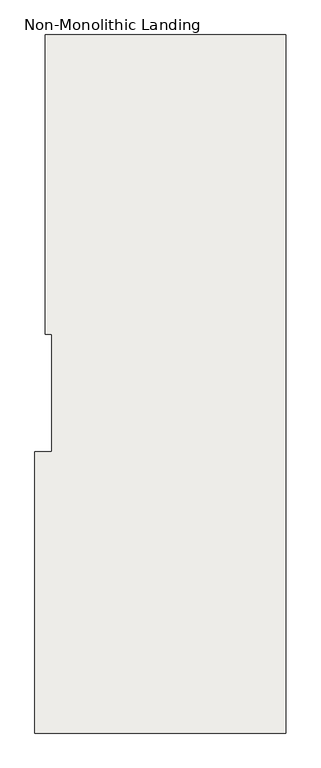
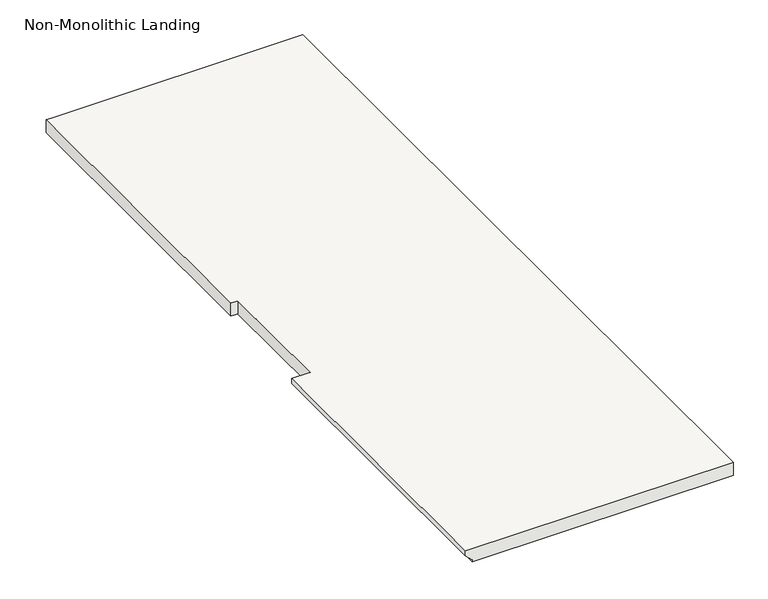
"""IFC4 building model written with IfcOpenShell, lengths in millimetres: slab geometry, Non-Monolithic Landing."""

from ifc_helpers import new_model, si_unit, origin, place, context, project, spatial, faceted_brep, source, transform, mapped, element, save


def non_monolithic_landing_4509e35c(model_context):
    return source(origin(), model_context, "Body", "Brep", [
        faceted_brep([(-1773.5888787, 2474.8939653, 996.95), (-1773.5888787, 2474.8939653, 1016.0), (-1773.5888787, 3576.1973029, 1016.0), (-1773.5888787, 3576.1973029, 996.95), (-1748.1888787, 2474.8939653, 971.55), (-1748.1888787, 3576.1973029, 971.55), (-792.3886283, 2474.8939653, 1016.0), (-792.3886283, 5206.8078573, 1016.0), (-1706.7886283, 5206.8078573, 1016.0), (-1732.1886283, 5206.8078573, 1016.0), (-1732.1886283, 4034.5574946, 1016.0), (-1706.7886283, 4034.5574946, 1016.0), (-1706.7886283, 3576.1973029, 1016.0), (-1748.1888787, 2474.8939653, 965.2), (-1748.1888787, 3576.1973029, 965.2), (-1706.7886283, 3576.1973029, 965.2), (-1706.7886283, 4034.5574946, 965.2), (-1732.1886283, 4034.5574946, 965.2), (-1732.1886283, 5206.8078573, 965.2), (-1706.7886283, 5206.8078573, 965.2), (-792.3886283, 5206.8078573, 965.2), (-792.3886283, 2474.8939653, 965.2)], [[[0, 1, 2, 3]], [[4, 0, 3, 5]], [[6, 7, 8, 9, 10, 11, 12, 2, 1]], [[13, 14, 15, 16, 17, 18, 19, 20, 21]], [[14, 13, 4, 5]], [[6, 1, 0, 4, 13, 21]], [[7, 6, 21, 20]], [[8, 7, 20, 19]], [[9, 8, 19, 18]], [[10, 9, 18, 17]], [[11, 10, 17, 16]], [[12, 11, 16, 15]], [[2, 12, 15, 14, 5, 3]]]),
    ])


if __name__ == "__main__":
    model = new_model("IFC4")
    model_context = context("Model", 3, world=origin())
    ifc_project = project(units=[si_unit("LENGTHUNIT", "METRE", prefix="MILLI")], contexts=[model_context])
    site = spatial("IfcSite", under=ifc_project)
    building = spatial("IfcBuilding", under=site)
    placement = place(None, origin())
    non_monolithic_landing_shape = non_monolithic_landing_4509e35c(model_context)
    element("IfcSlab", 1, ObjectType="Non-Monolithic Landing", at=placement, inside=building, context=model_context, shape_type="MappedRepresentation", body=[
        mapped(non_monolithic_landing_shape, transform((0.0, 0.0, 0.0), x_axis=(1.0, 0.0, 0.0), y_axis=(0.0, 1.0, 0.0), z_axis=(0.0, 0.0, 1.0))),
    ])
    save(model, "model.ifc")
